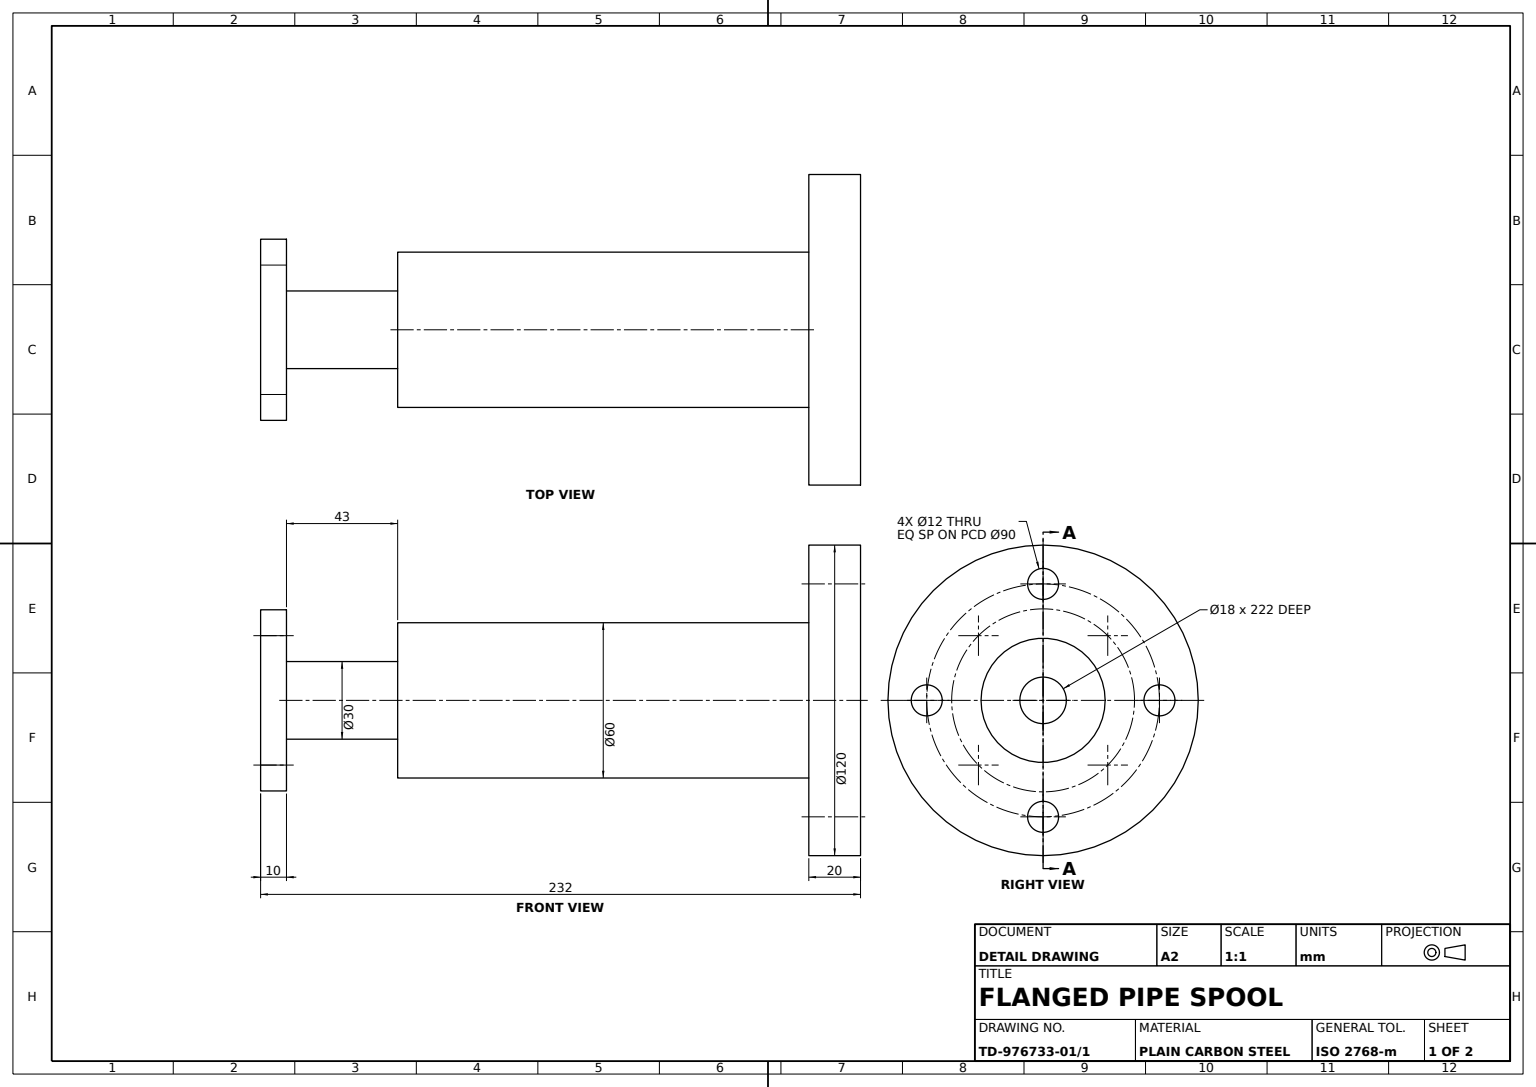
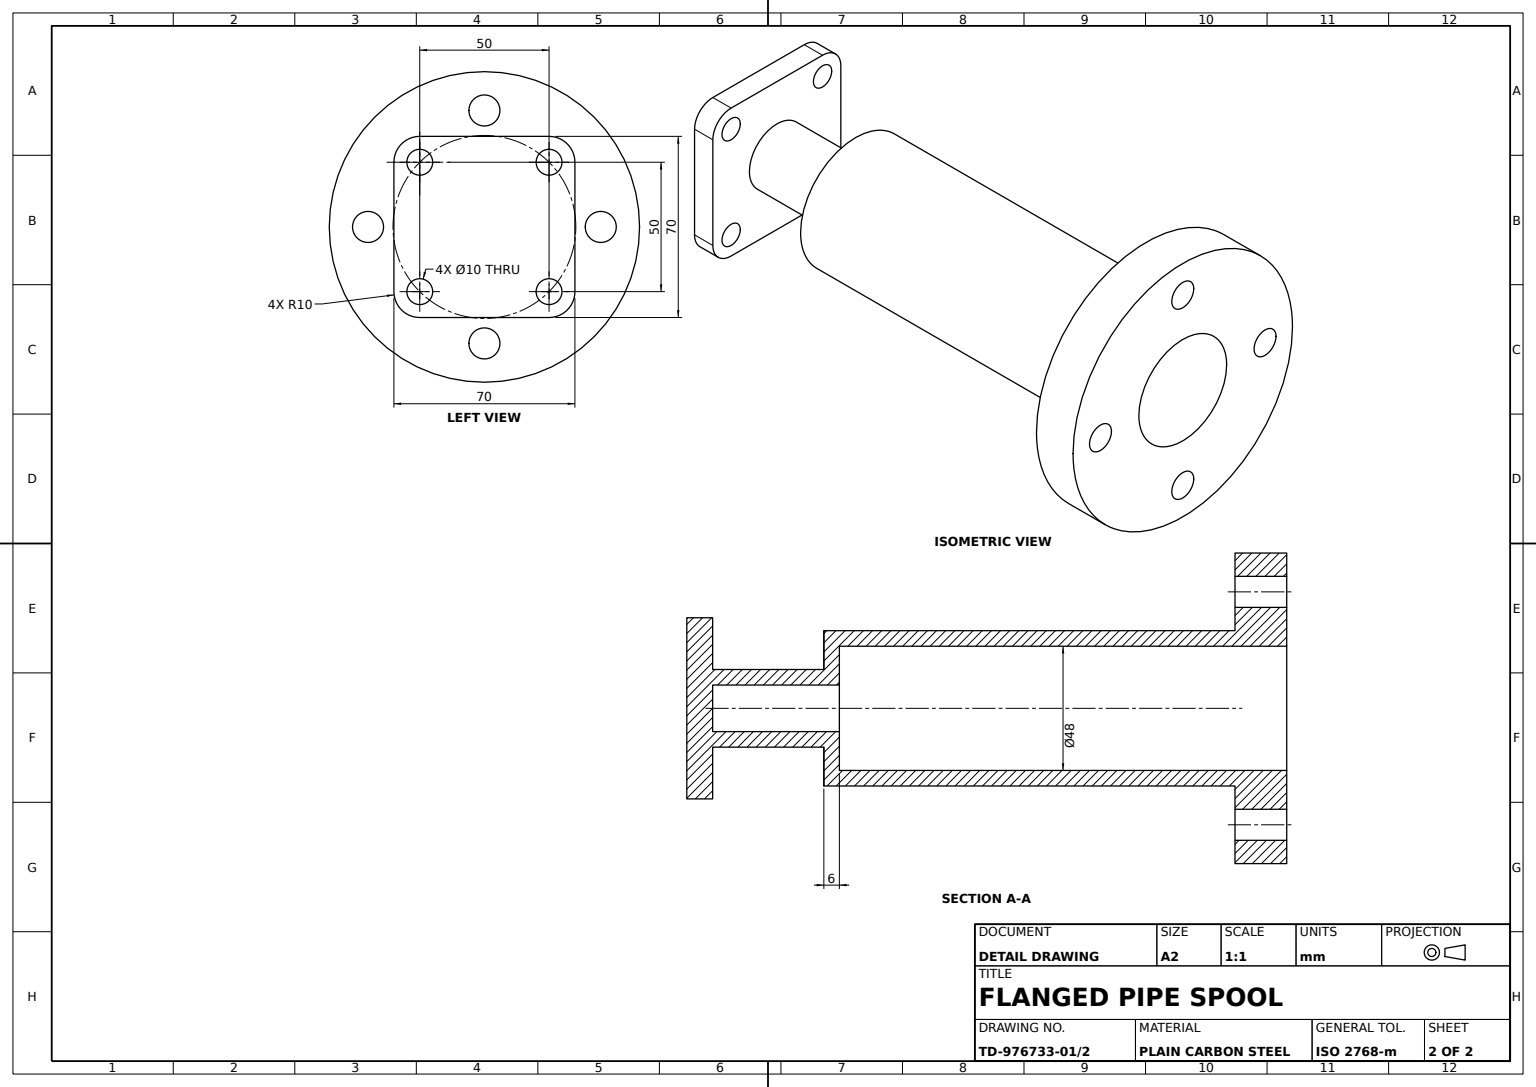
from build123d import *

# Parameters (mm, degrees)
SQUARE_FLANGE_SKETCH_70X70_W            = 70
SQUARE_FLANGE_SKETCH_70X70_H            = 70
SQUARE_MOUNTING_FLANGE_DEPTH            = 10
SQUARE_FLANGE_CORNER_FILLETS_R10_R      = 10
SQUARE_FLANGE_HOLES_SKETCH_R            = 5
SQUARE_FLANGE_MOUNTING_HOLES_4X_DEPTH   = 10
ROUND_FLANGE_HOLE_SKETCH_R              = 6
ROUND_FLANGE_BOLT_HOLE_12_DEPTH         = 229.350607619
ROUND_FLANGE_BOLT_HOLE_PATTERN_4X_COUNT = 4


with BuildPart() as part:
    # Housing Profile Sketch → Housing Body Revolve (revolve)
    with BuildSketch(Plane.XY, mode=Mode.PRIVATE) as housing_body_revolve_sk:
        Polygon((0, 15), (43, 15), (43, 30), (202, 30), (202, 60), (222, 60), (222, 24), (49, 24), (49, 9), (0, 9), align=None)
    revolve(housing_body_revolve_sk.sketch.rotate(Axis((0, 0, 0), (1, 0, 0)), 90), axis=Axis((0, 0, 0), (1, 0, 0)))

    # Square Flange Sketch 70x70 → Square Mounting Flange (add)
    with BuildSketch(Plane.ZY):
        Rectangle(SQUARE_FLANGE_SKETCH_70X70_W, SQUARE_FLANGE_SKETCH_70X70_H)
    extrude(amount=SQUARE_MOUNTING_FLANGE_DEPTH)

    # Square Flange Corner Fillets R10
    square_flange_corner_fillets_r10_edges = [part.edges().sort_by_distance(p)[0] for p in [
        (-5, -35, 35),
        (-5, 35, 35),
        (-5, 35, -35),
        (-5, -35, -35),
    ]]
    fillet(square_flange_corner_fillets_r10_edges, radius=SQUARE_FLANGE_CORNER_FILLETS_R10_R)

    # Square Flange Holes Sketch → Square Flange Mounting Holes 4x (cut)
    with BuildSketch(Plane.ZY.offset(10)):
        with Locations((25, 25)):
            Circle(SQUARE_FLANGE_HOLES_SKETCH_R)
        with Locations((-25, 25)):
            Circle(SQUARE_FLANGE_HOLES_SKETCH_R)
        with Locations((-25, -25)):
            Circle(SQUARE_FLANGE_HOLES_SKETCH_R)
        with Locations((25, -25)):
            Circle(SQUARE_FLANGE_HOLES_SKETCH_R)
    extrude(amount=-SQUARE_FLANGE_MOUNTING_HOLES_4X_DEPTH, mode=Mode.SUBTRACT)

    # Round Flange Hole Sketch → Round Flange Bolt Hole Ø12 (cut, through all)
    with BuildSketch(Plane.ZY.offset(-202)):
        with Locations((45, 0)):
            Circle(ROUND_FLANGE_HOLE_SKETCH_R)
    round_flange_bolt_hole_12 = extrude(amount=-ROUND_FLANGE_BOLT_HOLE_12_DEPTH, mode=Mode.SUBTRACT)

    # Round Flange Bolt Hole Pattern 4x: Round Flange Bolt Hole Ø12 ×4 about axis
    round_flange_bolt_hole_pattern_4x_axis = Axis((0, 0, 0), (1, 0, 0))
    for i in range(1, ROUND_FLANGE_BOLT_HOLE_PATTERN_4X_COUNT):
        add(round_flange_bolt_hole_12.rotate(round_flange_bolt_hole_pattern_4x_axis, i * 360 / ROUND_FLANGE_BOLT_HOLE_PATTERN_4X_COUNT), mode=Mode.SUBTRACT)


solid = part.part
